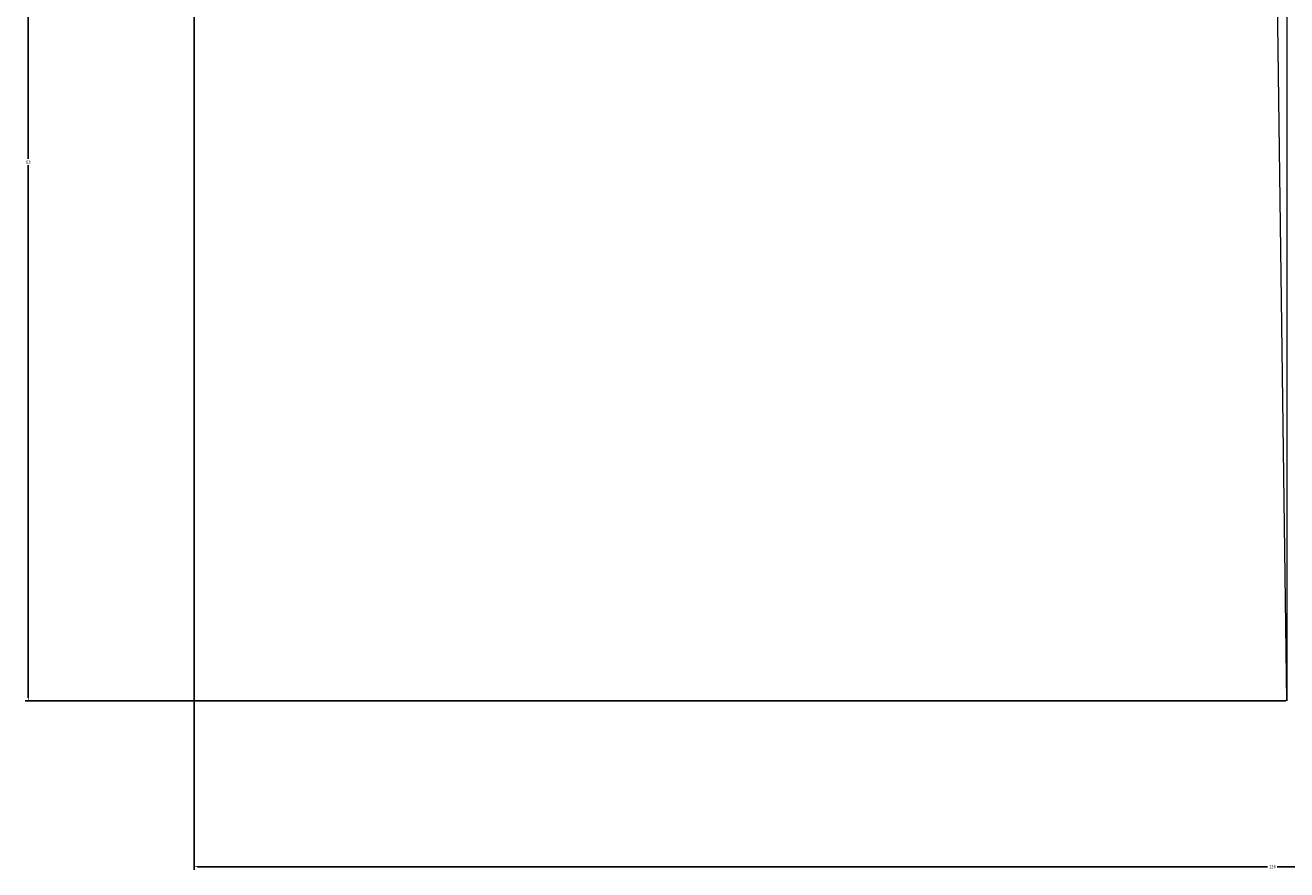
# Model space of a CAD drawing. Units: millimetres. Extents: x -136 to 10, y 158 to 257.
# Tile 1 of 6: x -136 to -62, y 158 to 208. Entities that reach past the tile are written whole.
import ezdxf

# ---------------------------------------------------------------- set-up
doc = ezdxf.new("R2010")
doc.units = ezdxf.units.MM
doc.layers.add('M-CONS', color=8, linetype='Continuous', lineweight=18)
doc.layers.add('M-DIMS', color=2, linetype='Continuous', lineweight=18)
doc.styles.get("Standard").update_dxf_attribs({"font": 'arial.ttf'})
doc.dimstyles.get("Standard").update_dxf_attribs({"dimtxt": 0.18, "dimasz": 0.18, "dimexe": 0.18, "dimexo": 0.0625, "dimgap": 0.09, "dimtad": 0, "dimtih": 1, "dimtoh": 1, "dimdec": 4, "dimzin": 0, "dimdsep": 46, "dimtxsty": 'Standard', "dimcen": 0.09, "dimadec": 0, "dimazin": 0, "dimtfac": 1, "dimtdec": 4, "dimtofl": 0, "dimtmove": 0, "dimatfit": 3, "dimfxl": 1, "dimtolj": 1, "dimtzin": 0, "dimarcsym": 0})

# ---------------------------------------------------------------- blocks, each defined once
blk = doc.blocks.new('*D1')
at = {"layer": 'Defpoints', "color": 0, "transparency": 16777216}
for p in [(-126, 231.107), (0, 231.107), (0, 158.407)]:
    blk.add_point(p, dxfattribs=at)
at = {"layer": 'M-DIMS', "color": 0, "lineweight": -2, "transparency": 16777216}
for p, q in [((-126, 231.044), (-126, 158.227)), ((0, 231.044), (0, 158.227)), ((-125.82, 158.407), (-63.28, 158.407)), ((-0.18, 158.407), (-62.72, 158.407))]:
    blk.add_line(p, q, dxfattribs=at)
at = {"layer": 'M-DIMS', "color": 0, "transparency": 16777216}
for points in [[(-125.82, 158.437), (-125.82, 158.377), (-126, 158.407)], [(-0.18, 158.437), (-0.18, 158.377), (0, 158.407)]]:
    blk.add_solid(points, dxfattribs=at)
at = {"layer": 'M-DIMS', "color": 0, "transparency": 16777216, "insert": (-63, 158.407), "char_height": 0.18, "attachment_point": 5}
blk.add_mtext('\\A1;126', dxfattribs=at)
blk = doc.blocks.new('*D3')
at = {"layer": 'Defpoints', "color": 0, "transparency": 16777216}
for p in [(-126, 231.107), (-135.7, 168.107), (-62.158, 168.107)]:
    blk.add_point(p, dxfattribs=at)
at = {"layer": 'M-DIMS', "color": 0, "lineweight": -2, "transparency": 16777216}
for p, q in [((-126.062, 231.107), (-135.88, 231.107)), ((-135.7, 230.927), (-135.7, 199.789)), ((-135.7, 168.287), (-135.7, 199.425)), ((-62.22, 168.107), (-135.88, 168.107))]:
    blk.add_line(p, q, dxfattribs=at)
at = {"layer": 'M-DIMS', "color": 0, "transparency": 16777216}
for points in [[(-135.73, 230.927), (-135.67, 230.927), (-135.7, 231.107)], [(-135.73, 168.287), (-135.67, 168.287), (-135.7, 168.107)]]:
    blk.add_solid(points, dxfattribs=at)
at = {"layer": 'M-DIMS', "color": 0, "transparency": 16777216, "insert": (-135.7, 199.607), "char_height": 0.18, "attachment_point": 5}
blk.add_mtext('\\A1;63', dxfattribs=at)

msp = doc.modelspace()

# ---------------------------------------------------------------- linework, layer by layer
at = {"layer": 'M-CONS'}
msp.add_polyline3d([(-62.158, 168.1068, 112.8035), (-63, 231.1068, 68.8035), (-62.158, 231.1068, 112.8035)], close=True, dxfattribs=at)

# ---------------------------------------------------------------- dimensions: what is measured, and where the dimension line sits
at = {"layer": 'M-DIMS'}
dim = msp.add_linear_dim(base=(-135.7, 168.1068), p1=(-126, 231.1068), p2=(-62.158, 168.1068), angle=90, dimstyle='Standard', override={"dimdec": 0, "dimlfac": 1, "dimrnd": 0, "dimzin": 0, "dimdsep": 46, "dimlunit": 2}, dxfattribs=at)
dim.commit()
dim.dimension.update_dxf_attribs({"geometry": '*D3', "text_midpoint": (-135.7, 199.6068)})
dim = msp.add_linear_dim(base=(0, 158.4068), p1=(-126, 231.1068), p2=(0, 231.1068), dimstyle='Standard', override={"dimdec": 0, "dimlfac": 1, "dimrnd": 0, "dimzin": 0, "dimdsep": 46, "dimlunit": 2}, dxfattribs=at)
dim.commit()
dim.dimension.update_dxf_attribs({"geometry": '*D1', "text_midpoint": (-63, 158.4068)})

doc.saveas('drawing.dxf')
